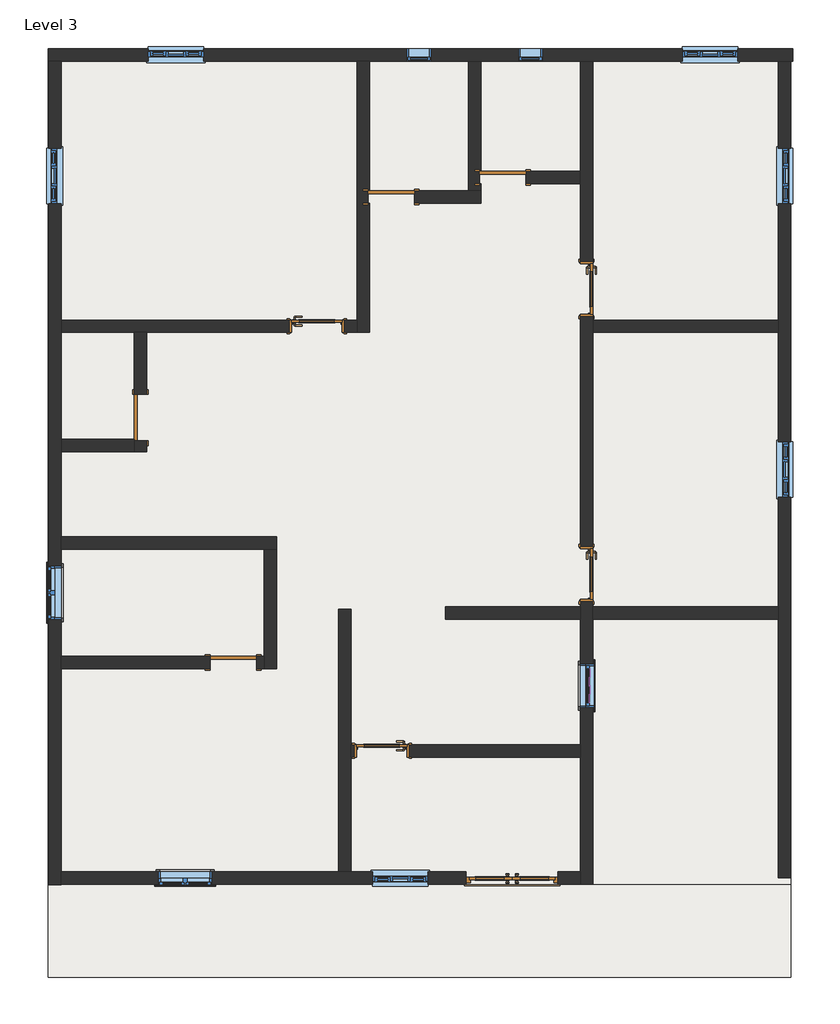
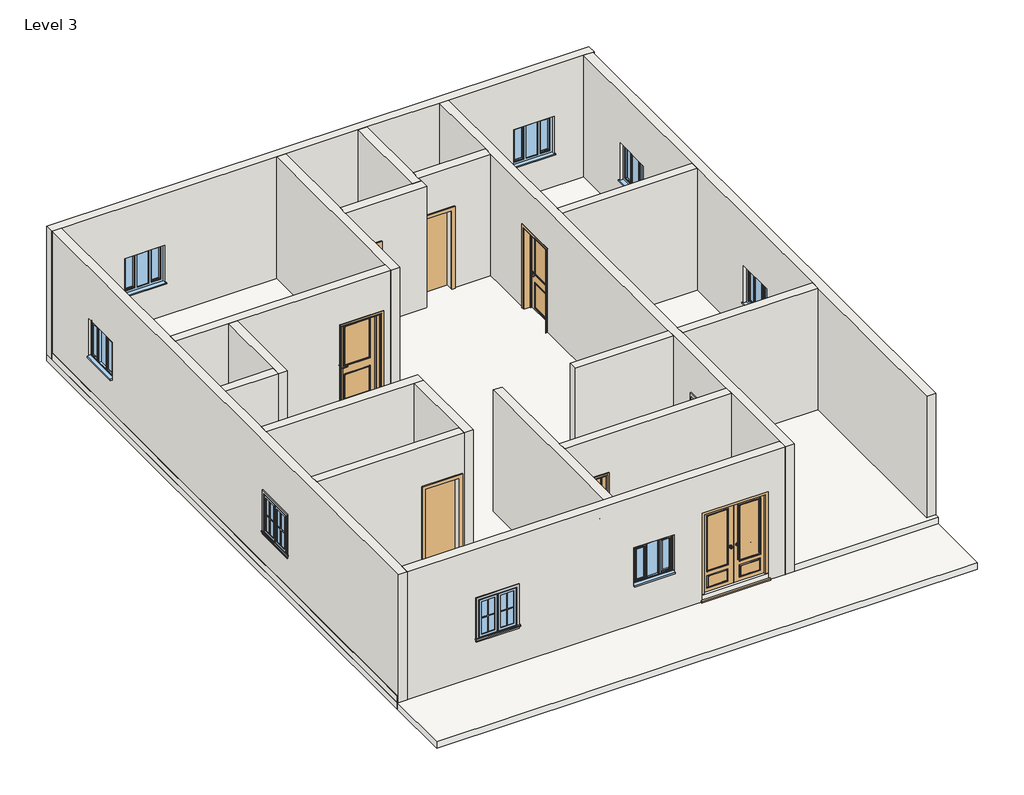
# One storey, incomplete: 19 walls, 12 proxies, 11 windows, 9 doors, 2 slabs, 1 roof.
# Revit data of these elements (continued)
# Element 34 (IfcWall, "4.5\" p") (continued)
#   wall height = 10' - 0"
#   Phase Created = New Construction
#   Base Constraint = Level 3
#   Top Constraint = Level 4
#   Materials on its faces: "Default Wall", "Render Material 255-0-255"
# Element 40 (IfcWall, "9\"")
#   Top Offset = 0' - 0"
#   Base Offset = 0' - 0"
#   wall height = 10' - 0"
#   Phase Created = New Construction
#   Base Constraint = Level 3
#   Top Constraint = Level 4
#   Materials on its faces: "Default Wall"
# Elements 41, 42 (IfcWall, "9\" wall")
#   Top Offset = 0' - 0"
#   Base Offset = 0' - 0"
#   wall height = 10' - 0"
#   Phase Created = New Construction
#   Base Constraint = Level 3
#   Top Constraint = Level 4
#   Materials on its faces: "Default Wall"
# Element 43 (IfcWall, "9\" wall")
#   Top Offset = 0' - 0"
#   Base Offset = 0' - 0"
#   wall height = 10' - 0"
#   Phase Created = New Construction
#   Base Constraint = Level 3
#   Top Constraint = Level 4
#   Materials on its faces: "Default Wall", "Render Material 255-0-255"
# Element 44 (IfcWindow, "Fixed : 16\" x 24\"")
#   Mark = "31"
#   Phase Created = New Construction
#   Materials on its faces: "Sash", "Glass"
# Element 45 (IfcWindow, "Fixed : 16\" x 24\"")
#   Mark = "32"
#   Phase Created = New Construction
#   Materials on its faces: "Sash", "Glass"
# Element 46 (IfcWindow, "Window-Casement-Double : 34\" x 36\"")
#   Mark = "23"
#   Window Inset = 0' - 0"
#   Interior Wall Closure = 0' - 2 1/4"
#   Frame Extension = 0' - 0 1/4"
#   Exterior Wall Closure = 0' - 1 1/4"
#   Interior Trim Visibility = yes
#   Exterior Trim Visibility = yes
#   Phase Created = New Construction
#   Materials on its faces: "Wood - Stained", "Glass", "Clad - White"
# Element 47 (IfcWindow, "Window-Casement-Double : 34\" x 36\"")
#   Mark = "24"
#   Window Inset = 0' - 0"
#   Interior Wall Closure = 0' - 2 1/4"
#   Frame Extension = 0' - 0 1/4"
#   Exterior Wall Closure = 0' - 1 1/4"
#   Interior Trim Visibility = yes
#   Exterior Trim Visibility = yes
#   Phase Created = New Construction
#   Materials on its faces: "Wood - Stained", "Glass", "Clad - White"
# Element 48 (IfcWindow, "Window-Double-Hung : 28\" x 46\"")
#   Mark = "33"
#   Window Inset = 0' - 0"
#   Interior Wall Closure = 0' - 1 1/2"
#   Frame Extension = 0' - 1 1/4"
#   Exterior Wall Closure = 0' - 0 1/2"
#   Interior Trim Visibility = yes
#   Indicator Visibility = yes
#   Exterior Trim Visibility = yes
#   Phase Created = New Construction
#   Materials on its faces: "Wood - Stained", "Glass", "Clad - White"
# Element 49 (IfcWindow, "Windows_Tpl_Plain : 910x910mm")
#   Mark = "25"
#   Phase Created = New Construction
#   Materials on its faces: "Window Frame", "Glass"
# Element 50 (IfcWindow, "Windows_Tpl_Plain : 910x910mm")
#   Mark = "28"
#   Phase Created = New Construction
#   Materials on its faces: "Window Frame", "Glass"
# Element 51 (IfcWindow, "Windows_Tpl_Plain : 910x910mm")
#   Mark = "29"
#   Phase Created = New Construction
#   Materials on its faces: "Window Frame", "Glass"
# Element 52 (IfcWindow, "Windows_Tpl_Plain : 910x910mm")
#   Mark = "30"
#   Phase Created = New Construction
#   Materials on its faces: "Window Frame", "Glass"
# Element 53 (IfcWindow, "Windows_Tpl_Plain : 910x910mm")
#   Mark = "26"
#   Phase Created = New Construction
#   Materials on its faces: "Window Frame", "Glass"
# Element 54 (IfcWindow, "Windows_Tpl_Plain : 910x910mm")
#   Mark = "27"
#   Phase Created = New Construction
#   Materials on its faces: "Window Frame", "Glass"
# Materials
#   "Door - Panel": class "Wood", colour RGB 210 159 95, transparency 0, Cost = 0
#   "Door - Glazing": colour RGB 0 0 255, transparency 0.75
#   "Door - Frame/Mullion": class "Wood", colour RGB 212 179 113, transparency 0
#   "Door - Handle": colour RGB 247 247 247, transparency 0
#   "Door - Architrave": class "Wood", colour RGB 154 90 5, transparency 0
#   "Door - Frame": colour RGB 118 70 51, transparency 0, Cost = 0
#   "Glass": class "Glass", colour RGB 0 128 192, transparency 0.75, Description = "Soda Lime Glass", Cost = 0
#   "Sash": class "Wood", colour RGB 224 178 126, transparency 0, Cost = 0
#   "Wood - Stained": class "Wood", colour RGB 224 178 126, transparency 0, Cost = 0
#   "Clad - White": class "Wood", colour RGB 242 242 238, transparency 0, Cost = 0
#   "Window Frame": colour RGB 249 249 249, transparency 0
#   "Default Roof": colour RGB 88 101 114, transparency 0, Cost = 0
#   "Default Floor": colour RGB 128 128 128, transparency 0, Cost = 0
#   "Default Wall": colour RGB 128 128 128, transparency 0, Cost = 0
#   "Render Material 255-0-255": colour RGB 255 0 255, transparency 0
